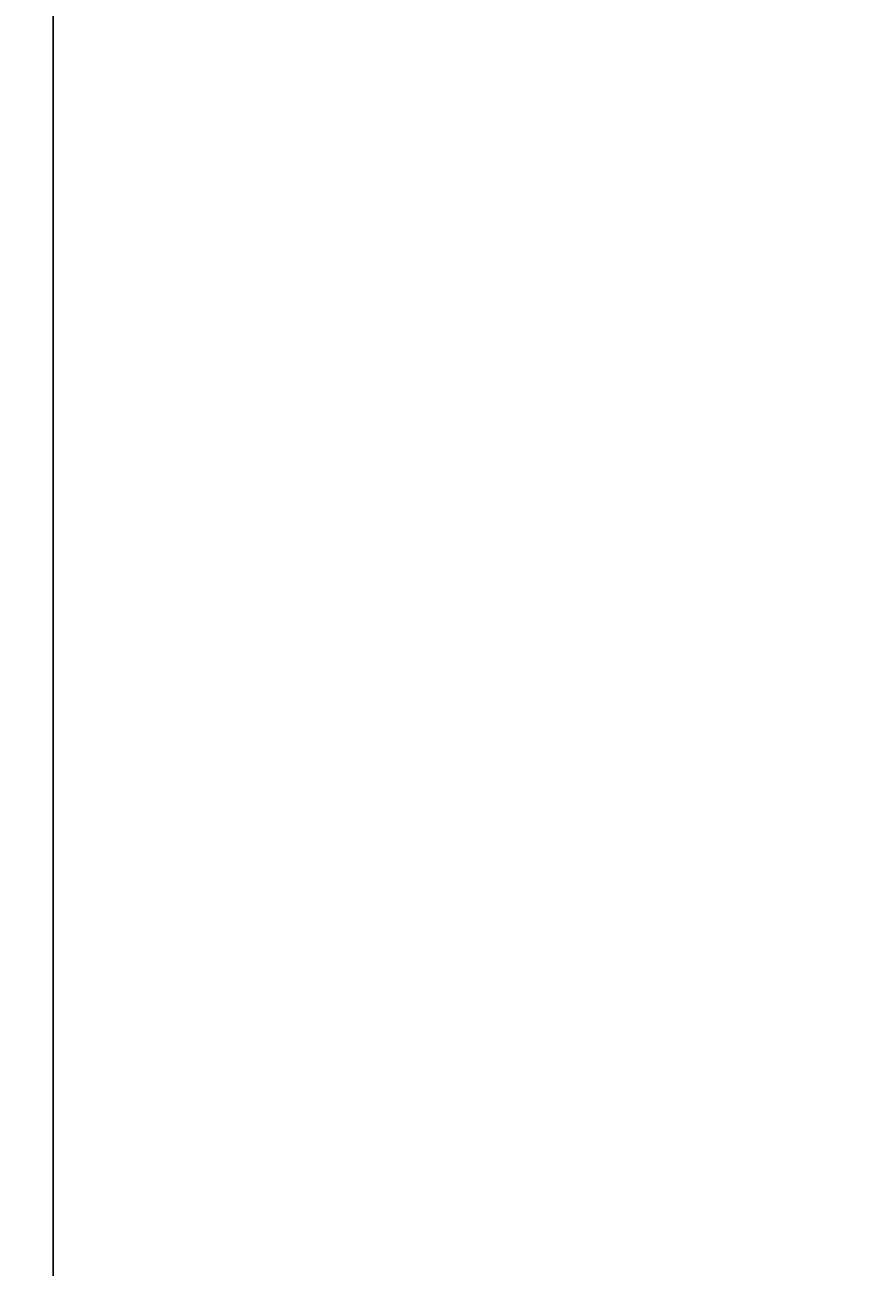
# Model space of a CAD drawing. Units: millimetres. Extents: x 27017497 to 27018854, y 7058029 to 7059154.
# Tile 3 of 91: x 27017560 to 27017605, y 7058133 to 7058200. Entities that reach past the tile are written whole.
import ezdxf

# ---------------------------------------------------------------- set-up
doc = ezdxf.new("R2010")
doc.units = ezdxf.units.MM
doc.layers.add('A-ANNO-DIMS', color=2, linetype='Continuous', lineweight=18)
doc.styles.get("Standard").update_dxf_attribs({"font": 'arial.ttf'})
doc.dimstyles.get("Standard").update_dxf_attribs({"dimtxt": 0.18, "dimasz": 0.18, "dimexe": 0.18, "dimexo": 0.0625, "dimgap": 0.09, "dimtad": 0, "dimtih": 1, "dimtoh": 1, "dimdec": 4, "dimzin": 0, "dimdsep": 46, "dimtxsty": 'Standard', "dimcen": 0.09, "dimadec": 0, "dimazin": 0, "dimtfac": 1, "dimtdec": 4, "dimtofl": 0, "dimtmove": 0, "dimatfit": 3, "dimfxl": 1, "dimtolj": 1, "dimtzin": 0, "dimarcsym": 0})

# ---------------------------------------------------------------- blocks, each defined once
blk = doc.blocks.new('*D47')
at = {"layer": 'A-ANNO-DIMS', "color": 0, "lineweight": -2, "transparency": 16777216}
for p, q in [((27017561.166, 7058294.35), (27017561.166, 7058028.6)), ((27018790.606, 7058294.35), (27018790.606, 7058028.6)), ((27017561.346, 7058028.78), (27018175.431, 7058028.78)), ((27018790.426, 7058028.78), (27018176.341, 7058028.78))]:
    blk.add_line(p, q, dxfattribs=at)
at = {"layer": 'A-ANNO-DIMS', "color": 0, "transparency": 16777216}
for points in [[(27017561.346, 7058028.81), (27017561.346, 7058028.75), (27017561.166, 7058028.78)], [(27018790.426, 7058028.81), (27018790.426, 7058028.75), (27018790.606, 7058028.78)]]:
    blk.add_solid(points, dxfattribs=at)
at = {"layer": 'Defpoints', "color": 0, "transparency": 16777216}
for p in [(27017561.166, 7058294.412), (27018790.606, 7058294.412), (27018790.606, 7058028.78)]:
    blk.add_point(p, dxfattribs=at)
at = {"layer": 'A-ANNO-DIMS', "color": 0, "transparency": 16777216, "insert": (27018175.886, 7058028.78), "char_height": 0.18, "attachment_point": 5}
blk.add_mtext('\\A1;1229.4', dxfattribs=at)
blk = doc.blocks.new('*D48')
at = {"layer": 'A-ANNO-DIMS', "color": 0, "lineweight": -2, "transparency": 16777216}
for p, q in [((27018463.498, 7058622.912), (27017497.536, 7058622.912)), ((27017497.716, 7058622.732), (27017497.716, 7058357.753)), ((27017497.716, 7058092.41), (27017497.716, 7058357.389)), ((27018555.129, 7058092.23), (27017497.536, 7058092.23))]:
    blk.add_line(p, q, dxfattribs=at)
at = {"layer": 'A-ANNO-DIMS', "color": 0, "transparency": 16777216}
for points in [[(27017497.686, 7058622.732), (27017497.746, 7058622.732), (27017497.716, 7058622.912)], [(27017497.686, 7058092.41), (27017497.746, 7058092.41), (27017497.716, 7058092.23)]]:
    blk.add_solid(points, dxfattribs=at)
at = {"layer": 'Defpoints', "color": 0, "transparency": 16777216}
for p in [(27018463.561, 7058622.912), (27017497.716, 7058092.23), (27018555.192, 7058092.23)]:
    blk.add_point(p, dxfattribs=at)
at = {"layer": 'A-ANNO-DIMS', "color": 0, "transparency": 16777216, "insert": (27017497.716, 7058357.571), "char_height": 0.18, "attachment_point": 5}
blk.add_mtext('\\A1;530.7', dxfattribs=at)

msp = doc.modelspace()

# ---------------------------------------------------------------- dimensions: what is measured, and where the dimension line sits
at = {"layer": 'A-ANNO-DIMS'}
dim = msp.add_linear_dim(base=(27017497.716, 7058092.23), p1=(27018463.561, 7058622.912), p2=(27018555.192, 7058092.23), angle=90, dimstyle='Standard', override={"dimdec": 1, "dimlfac": 1, "dimrnd": 0, "dimzin": 0, "dimdsep": 46, "dimlunit": 2}, dxfattribs=at)
dim.commit()
dim.dimension.update_dxf_attribs({"geometry": '*D48', "text_midpoint": (27017497.716, 7058357.571)})
dim = msp.add_linear_dim(base=(27018790.606, 7058028.78), p1=(27017561.166, 7058294.412), p2=(27018790.606, 7058294.412), dimstyle='Standard', override={"dimdec": 1, "dimlfac": 1, "dimrnd": 0, "dimzin": 0, "dimdsep": 46, "dimlunit": 2}, dxfattribs=at)
dim.commit()
dim.dimension.update_dxf_attribs({"geometry": '*D47', "text_midpoint": (27018175.886, 7058028.78)})

doc.saveas('drawing.dxf')
